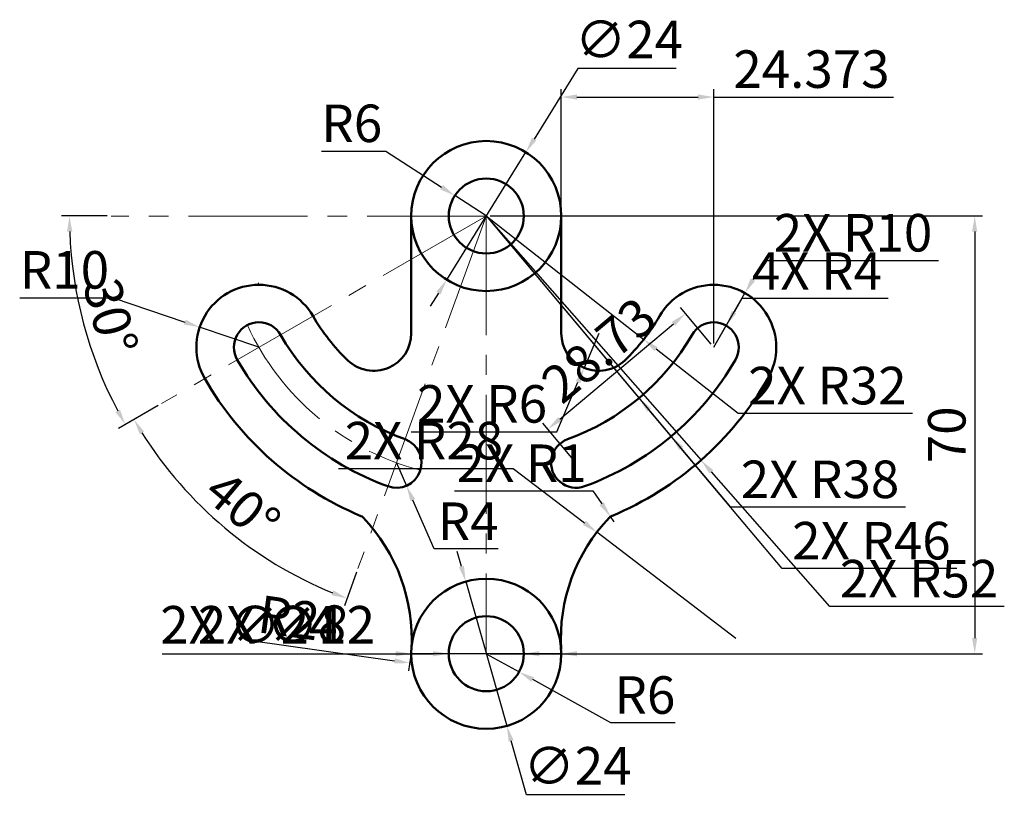
# Model space of a CAD drawing. Units: millimetres. Extents: x 1 to 158, y 37 to 161.
import ezdxf

# ---------------------------------------------------------------- set-up
doc = ezdxf.new("R2010")
doc.units = ezdxf.units.MM
doc.linetypes.add('CENTER2', pattern=[28.575, 19.05, -3.175, 3.175, -3.175])
for name, color, linetype, lineweight in [('M-CNTR', 4, 'CENTER2', 18), ('M-DIMS', 2, 'Continuous', 25), ('M-OUTL', 7, 'Continuous', 50)]:
    doc.layers.add(name, color=color, linetype=linetype, lineweight=lineweight)
doc.styles.get("Standard").update_dxf_attribs({"font": 'arial.ttf'})
doc.dimstyles.new('ISO-25', dxfattribs={"dimtxt": 6, "dimasz": 2.5, "dimexe": 1.25, "dimexo": 0.625, "dimtad": 1, "dimtoh": 1, "dimdec": 0, "dimtxsty": 'Standard', "dimcen": 2.5, "dimadec": 0, "dimazin": 0, "dimtfac": 1, "dimtdec": 0, "dimtmove": 0, "dimatfit": 3, "dimfxl": 1, "dimarcsym": 0})

# ---------------------------------------------------------------- blocks, each defined once
blk = doc.blocks.new('*D1')
at = {"layer": 'Defpoints', "color": 0, "transparency": 16777216}
for p in [(70.21, 133.22), (75.25, 129.97)]:
    blk.add_point(p, dxfattribs=at)
at = {"layer": 'M-DIMS', "color": 0, "lineweight": -2, "transparency": 16777216}
for p, q in [((48.9, 140.32), (59.2, 140.32)), ((59.2, 140.32), (68.11, 134.57)), ((75.25, 129.97), (70.21, 133.22))]:
    blk.add_line(p, q, dxfattribs=at)
at = {"layer": 'M-DIMS', "color": 0, "transparency": 16777216}
blk.add_solid([(68.34, 134.92), (67.89, 134.22), (70.21, 133.22)], dxfattribs=at)
at = {"layer": 'M-DIMS', "color": 0, "transparency": 16777216, "insert": (53.74, 144.01), "char_height": 6, "attachment_point": 5}
blk.add_mtext('R6', dxfattribs=at)
blk = doc.blocks.new('*D2')
at = {"layer": 'Defpoints', "color": 0, "transparency": 16777216}
for p in [(81.59, 140.16), (68.92, 119.77)]:
    blk.add_point(p, dxfattribs=at)
at = {"layer": 'M-DIMS', "color": 0, "lineweight": -2, "transparency": 16777216}
for p, q in [((89.91, 153.57), (82.9, 142.28)), ((105.64, 153.57), (89.91, 153.57)), ((68.92, 119.77), (81.59, 140.16)), ((67.6, 117.65), (66.29, 115.53))]:
    blk.add_line(p, q, dxfattribs=at)
at = {"layer": 'M-DIMS', "color": 0, "transparency": 16777216}
for points in [[(82.55, 142.5), (83.26, 142.06), (81.59, 140.16)], [(67.25, 117.87), (67.96, 117.43), (68.92, 119.77)]]:
    blk.add_solid(points, dxfattribs=at)
at = {"layer": 'M-DIMS', "color": 0, "transparency": 16777216, "insert": (98.09, 157.42), "char_height": 6, "attachment_point": 5}
blk.add_mtext('∅24', dxfattribs=at)
blk = doc.blocks.new('*D3')
at = {"layer": 'Defpoints', "color": 0, "transparency": 16777216}
for p in [(75.25, 129.97), (75.25, 59.97), (153.37, 59.97)]:
    blk.add_point(p, dxfattribs=at)
at = {"layer": 'M-DIMS', "color": 0, "lineweight": -2, "transparency": 16777216}
for p, q in [((75.88, 129.97), (154.62, 129.97)), ((153.37, 127.47), (153.37, 62.47)), ((75.88, 59.97), (154.62, 59.97))]:
    blk.add_line(p, q, dxfattribs=at)
at = {"layer": 'M-DIMS', "color": 0, "transparency": 16777216}
for points in [[(152.95, 127.47), (153.78, 127.47), (153.37, 129.97)], [(152.95, 62.47), (153.78, 62.47), (153.37, 59.97)]]:
    blk.add_solid(points, dxfattribs=at)
at = {"layer": 'M-DIMS', "color": 0, "transparency": 16777216, "insert": (149.68, 94.97), "char_height": 6, "attachment_point": 5, "rotation": 90}
blk.add_mtext('70', dxfattribs=at)
blk = doc.blocks.new('*D4')
at = {"layer": 'Defpoints', "color": 0, "transparency": 16777216}
for p in [(35.33, 62.38), (63.05, 58.48)]:
    blk.add_point(p, dxfattribs=at)
at = {"layer": 'M-DIMS', "color": 0, "lineweight": -2, "transparency": 16777216}
blk.add_line((37.6, 62.06), (60.58, 58.82), dxfattribs=at)
blk.add_arc((35.33, 62.38), 28, 349.422, 355.2587, dxfattribs=at)
at = {"layer": 'M-DIMS', "color": 0, "transparency": 16777216}
blk.add_solid([(60.64, 59.24), (60.52, 58.41), (63.05, 58.48)], dxfattribs=at)
at = {"layer": 'M-DIMS', "color": 0, "transparency": 16777216, "insert": (45.84, 64.63), "char_height": 6, "attachment_point": 5, "rotation": 351.9799}
blk.add_mtext('R28', dxfattribs=at)
blk = doc.blocks.new('*D5')
at = {"layer": 'Defpoints', "color": 0, "transparency": 16777216}
for p in [(29.41, 112.19), (38.88, 108.97)]:
    blk.add_point(p, dxfattribs=at)
at = {"layer": 'M-DIMS', "color": 0, "lineweight": -2, "transparency": 16777216}
for p, q in [((0.63, 116.9), (15.57, 116.9)), ((15.57, 116.9), (27.05, 112.99)), ((38.88, 108.97), (29.41, 112.19))]:
    blk.add_line(p, q, dxfattribs=at)
at = {"layer": 'M-DIMS', "color": 0, "transparency": 16777216}
blk.add_solid([(27.18, 113.39), (26.91, 112.6), (29.41, 112.19)], dxfattribs=at)
at = {"layer": 'M-DIMS', "color": 0, "transparency": 16777216, "insert": (7.79, 120.58), "char_height": 6, "attachment_point": 5}
blk.add_mtext('R10', dxfattribs=at)
blk = doc.blocks.new('*D6')
at = {"layer": 'Defpoints', "color": 0, "transparency": 16777216}
for p in [(60.89, 90.5), (62.49, 86.83)]:
    blk.add_point(p, dxfattribs=at)
at = {"layer": 'M-DIMS', "color": 0, "lineweight": -2, "transparency": 16777216}
for p, q in [((60.89, 90.5), (62.49, 86.83)), ((66.9, 76.76), (63.5, 84.54)), ((77.18, 76.76), (66.9, 76.76))]:
    blk.add_line(p, q, dxfattribs=at)
at = {"layer": 'M-DIMS', "color": 0, "transparency": 16777216}
blk.add_solid([(63.88, 84.71), (63.11, 84.38), (62.49, 86.83)], dxfattribs=at)
at = {"layer": 'M-DIMS', "color": 0, "transparency": 16777216, "insert": (72.35, 80.38), "char_height": 6, "attachment_point": 5}
blk.add_mtext('R4', dxfattribs=at)
blk = doc.blocks.new('*D7')
at = {"layer": 'Defpoints', "color": 0, "transparency": 16777216}
for p in [(75.25, 129.97), (75.25, 129.97), (23.29, 99.97), (27.92, 85.31), (54.73, 73.58)]:
    blk.add_point(p, dxfattribs=at)
at = {"layer": 'M-DIMS', "color": 0, "lineweight": -2, "transparency": 16777216}
for p, q in [((22.75, 99.65), (17.81, 96.8)), ((54.52, 73), (52.57, 67.64))]:
    blk.add_line(p, q, dxfattribs=at)
blk.add_arc((75.25, 129.97), 65.08, 212.2012, 247.7988, dxfattribs=at)
at = {"layer": 'M-DIMS', "color": 0, "transparency": 16777216}
for points in [[(19.83, 95.07), (20.54, 95.5), (18.9, 97.43)], [(50.81, 70.1), (50.51, 69.33), (53, 68.81)]]:
    blk.add_solid(points, dxfattribs=at)
at = {"layer": 'M-DIMS', "color": 0, "transparency": 16777216, "insert": (35.79, 82.94), "char_height": 6, "attachment_point": 5, "rotation": 320}
blk.add_mtext('40°', dxfattribs=at)
blk = doc.blocks.new('*D8')
at = {"layer": 'Defpoints', "color": 0, "transparency": 16777216}
for p in [(15.25, 129.97), (75.25, 129.97), (75.25, 129.97), (9.6, 118.39), (23.29, 99.97)]:
    blk.add_point(p, dxfattribs=at)
at = {"layer": 'M-DIMS', "color": 0, "lineweight": -2, "transparency": 16777216}
for p, q in [((14.63, 129.97), (7.33, 129.97)), ((22.75, 99.65), (16.43, 96.01))]:
    blk.add_line(p, q, dxfattribs=at)
blk.add_arc((75.25, 129.97), 66.67, 182.1486, 207.8514, dxfattribs=at)
at = {"layer": 'M-DIMS', "color": 0, "transparency": 16777216}
for points in [[(8.21, 127.46), (9.05, 127.47), (8.58, 129.97)], [(16.67, 99.02), (15.94, 98.62), (17.52, 96.63)]]:
    blk.add_solid(points, dxfattribs=at)
at = {"layer": 'M-DIMS', "color": 0, "transparency": 16777216, "insert": (14.42, 113.67), "char_height": 6, "attachment_point": 5, "rotation": 285}
blk.add_mtext('30°', dxfattribs=at)
blk = doc.blocks.new('*D9')
at = {"layer": 'Defpoints', "color": 0, "transparency": 16777216}
for p in [(75.25, 59.97), (80.5, 57.05)]:
    blk.add_point(p, dxfattribs=at)
at = {"layer": 'M-DIMS', "color": 0, "lineweight": -2, "transparency": 16777216}
for p, q in [((75.25, 59.97), (80.5, 57.05)), ((95.16, 48.89), (82.68, 55.83)), ((105.46, 48.89), (95.16, 48.89))]:
    blk.add_line(p, q, dxfattribs=at)
at = {"layer": 'M-DIMS', "color": 0, "transparency": 16777216}
blk.add_solid([(82.88, 56.2), (82.48, 55.47), (80.5, 57.05)], dxfattribs=at)
at = {"layer": 'M-DIMS', "color": 0, "transparency": 16777216, "insert": (100.62, 52.58), "char_height": 6, "attachment_point": 5}
blk.add_mtext('R6', dxfattribs=at)
blk = doc.blocks.new('*D10')
at = {"layer": 'Defpoints', "color": 0, "transparency": 16777216}
for p in [(71.96, 71.51), (78.55, 48.43)]:
    blk.add_point(p, dxfattribs=at)
at = {"layer": 'M-DIMS', "color": 0, "lineweight": -2, "transparency": 16777216}
for p, q in [((71.28, 73.91), (70.59, 76.31)), ((71.96, 71.51), (78.55, 48.43)), ((81.69, 37.4), (79.23, 46.02)), ((97.41, 37.4), (81.69, 37.4))]:
    blk.add_line(p, q, dxfattribs=at)
at = {"layer": 'M-DIMS', "color": 0, "transparency": 16777216}
for points in [[(71.68, 74.02), (70.88, 73.8), (71.96, 71.51)], [(79.63, 46.14), (78.83, 45.91), (78.55, 48.43)]]:
    blk.add_solid(points, dxfattribs=at)
at = {"layer": 'M-DIMS', "color": 0, "transparency": 16777216, "insert": (89.86, 41.26), "char_height": 6, "attachment_point": 5}
blk.add_mtext('∅24', dxfattribs=at)
blk = doc.blocks.new('HUB-OD24-BORE12')
for radius in [12, 6]:
    blk.add_circle((12, 12), radius)
blk = doc.blocks.new('*D12')
at = {"layer": 'Defpoints', "color": 0, "transparency": 16777216}
for p in [(111.63, 148.99), (87.25, 111.2), (111.63, 108.97)]:
    blk.add_point(p, dxfattribs=at)
at = {"layer": 'M-DIMS', "color": 0, "lineweight": -2, "transparency": 16777216}
for p, q in [((87.25, 111.83), (87.25, 150.24)), ((111.63, 109.59), (111.63, 150.24)), ((89.75, 148.99), (109.13, 148.99)), ((111.63, 148.99), (140.39, 148.99))]:
    blk.add_line(p, q, dxfattribs=at)
at = {"layer": 'M-DIMS', "color": 0, "transparency": 16777216}
for points in [[(89.75, 149.41), (89.75, 148.57), (87.25, 148.99)], [(109.13, 149.41), (109.13, 148.57), (111.63, 148.99)]]:
    blk.add_solid(points, dxfattribs=at)
at = {"layer": 'M-DIMS', "color": 0, "transparency": 16777216, "insert": (127.26, 152.68), "char_height": 6, "attachment_point": 5}
blk.add_mtext('24.373', dxfattribs=at)
blk = doc.blocks.new('*D13')
at = {"layer": 'Defpoints', "color": 0, "transparency": 16777216}
for p in [(107.11, 114.35), (111.63, 108.97), (89.62, 90.5)]:
    blk.add_point(p, dxfattribs=at)
at = {"layer": 'M-DIMS', "color": 0, "lineweight": -2, "transparency": 16777216}
for p, q in [((111.23, 109.45), (106.31, 115.31)), ((87.02, 97.49), (105.2, 112.74)), ((89.22, 90.98), (84.3, 96.84))]:
    blk.add_line(p, q, dxfattribs=at)
at = {"layer": 'M-DIMS', "color": 0, "transparency": 16777216}
for points in [[(104.93, 113.06), (105.46, 112.42), (107.11, 114.35)], [(86.75, 97.81), (87.29, 97.17), (85.1, 95.88)]]:
    blk.add_solid(points, dxfattribs=at)
at = {"layer": 'M-DIMS', "color": 0, "transparency": 16777216, "insert": (93.74, 107.94), "char_height": 6, "attachment_point": 5, "rotation": 40}
blk.add_mtext('28.73', dxfattribs=at)
blk = doc.blocks.new('*D14')
at = {"layer": 'Defpoints', "color": 0, "transparency": 16777216}
for p in [(75.25, 129.97), (109.6, 90.92)]:
    blk.add_point(p, dxfattribs=at)
at = {"layer": 'M-DIMS', "color": 0, "lineweight": -2, "transparency": 16777216}
for p, q in [((75.25, 129.97), (109.6, 90.92)), ((130.21, 67.5), (111.25, 89.05)), ((158.1, 67.5), (130.21, 67.5))]:
    blk.add_line(p, q, dxfattribs=at)
at = {"layer": 'M-DIMS', "color": 0, "transparency": 16777216}
blk.add_solid([(111.57, 89.32), (110.94, 88.77), (109.6, 90.92)], dxfattribs=at)
at = {"layer": 'M-DIMS', "color": 0, "transparency": 16777216, "insert": (144.47, 71.19), "char_height": 6, "attachment_point": 5}
blk.add_mtext('2X R52', dxfattribs=at)
blk = doc.blocks.new('*D15')
at = {"layer": 'Defpoints', "color": 0, "transparency": 16777216}
for p in [(75.25, 129.97), (104.82, 94.73)]:
    blk.add_point(p, dxfattribs=at)
at = {"layer": 'M-DIMS', "color": 0, "lineweight": -2, "transparency": 16777216}
for p, q in [((75.25, 129.97), (104.82, 94.73)), ((122.56, 73.59), (106.43, 92.81)), ((150.52, 73.59), (122.56, 73.59))]:
    blk.add_line(p, q, dxfattribs=at)
at = {"layer": 'M-DIMS', "color": 0, "transparency": 16777216}
blk.add_solid([(106.75, 93.08), (106.11, 92.55), (104.82, 94.73)], dxfattribs=at)
at = {"layer": 'M-DIMS', "color": 0, "transparency": 16777216, "insert": (136.85, 77.27), "char_height": 6, "attachment_point": 5}
blk.add_mtext('2X R46', dxfattribs=at)
blk = doc.blocks.new('*D16')
at = {"layer": 'Defpoints', "color": 0, "transparency": 16777216}
for p in [(75.25, 129.97), (99.68, 100.86)]:
    blk.add_point(p, dxfattribs=at)
at = {"layer": 'M-DIMS', "color": 0, "lineweight": -2, "transparency": 16777216}
for p, q in [((75.25, 129.97), (99.68, 100.86)), ((114.34, 83.39), (101.29, 98.94)), ((142.3, 83.39), (114.34, 83.39))]:
    blk.add_line(p, q, dxfattribs=at)
at = {"layer": 'M-DIMS', "color": 0, "transparency": 16777216}
blk.add_solid([(101.61, 99.21), (100.97, 98.67), (99.68, 100.86)], dxfattribs=at)
at = {"layer": 'M-DIMS', "color": 0, "transparency": 16777216, "insert": (128.63, 87.08), "char_height": 6, "attachment_point": 5}
blk.add_mtext('2X R38', dxfattribs=at)
blk = doc.blocks.new('*D17')
at = {"layer": 'Defpoints', "color": 0, "transparency": 16777216}
for p in [(75.25, 129.97), (100.44, 110.22)]:
    blk.add_point(p, dxfattribs=at)
at = {"layer": 'M-DIMS', "color": 0, "lineweight": -2, "transparency": 16777216}
for p, q in [((75.25, 129.97), (100.44, 110.22)), ((115.55, 98.38), (102.41, 108.68)), ((143.44, 98.38), (115.55, 98.38))]:
    blk.add_line(p, q, dxfattribs=at)
at = {"layer": 'M-DIMS', "color": 0, "transparency": 16777216}
blk.add_solid([(102.66, 109.01), (102.15, 108.35), (100.44, 110.22)], dxfattribs=at)
at = {"layer": 'M-DIMS', "color": 0, "transparency": 16777216, "insert": (129.81, 102.07), "char_height": 6, "attachment_point": 5}
blk.add_mtext('2X R32', dxfattribs=at)
blk = doc.blocks.new('*D18')
at = {"layer": 'Defpoints', "color": 0, "transparency": 16777216}
for p in [(92.93, 79.38), (115.18, 62.38)]:
    blk.add_point(p, dxfattribs=at)
at = {"layer": 'M-DIMS', "color": 0, "lineweight": -2, "transparency": 16777216}
for p, q in [((51.61, 89.58), (79.58, 89.58)), ((79.58, 89.58), (90.94, 80.9)), ((115.18, 62.38), (92.93, 79.38))]:
    blk.add_line(p, q, dxfattribs=at)
at = {"layer": 'M-DIMS', "color": 0, "transparency": 16777216}
blk.add_solid([(91.2, 81.23), (90.69, 80.57), (92.93, 79.38)], dxfattribs=at)
at = {"layer": 'M-DIMS', "color": 0, "transparency": 16777216, "insert": (65.28, 93.27), "char_height": 6, "attachment_point": 5}
blk.add_mtext('2X R28', dxfattribs=at)
blk = doc.blocks.new('*D19')
at = {"layer": 'Defpoints', "color": 0, "transparency": 16777216}
for p in [(63.25, 59.97), (87.25, 59.97)]:
    blk.add_point(p, dxfattribs=at)
at = {"layer": 'M-DIMS', "color": 0, "lineweight": -2, "transparency": 16777216}
for p, q in [((23.39, 59.97), (51.79, 59.97)), ((51.79, 59.97), (60.75, 59.97)), ((87.25, 59.97), (63.25, 59.97)), ((89.75, 59.97), (92.25, 59.97))]:
    blk.add_line(p, q, dxfattribs=at)
at = {"layer": 'M-DIMS', "color": 0, "transparency": 16777216}
for points in [[(60.75, 60.38), (60.75, 59.55), (63.25, 59.97)], [(89.75, 60.38), (89.75, 59.55), (87.25, 59.97)]]:
    blk.add_solid(points, dxfattribs=at)
at = {"layer": 'M-DIMS', "color": 0, "transparency": 16777216, "insert": (37.28, 63.82), "char_height": 6, "attachment_point": 5}
blk.add_mtext('2X ∅24', dxfattribs=at)
blk = doc.blocks.new('*D20')
at = {"layer": 'Defpoints', "color": 0, "transparency": 16777216}
for p in [(69.25, 59.97), (81.25, 59.97)]:
    blk.add_point(p, dxfattribs=at)
at = {"layer": 'M-DIMS', "color": 0, "lineweight": -2, "transparency": 16777216}
for p, q in [((29.43, 59.97), (57.79, 59.97)), ((57.79, 59.97), (66.75, 59.97)), ((81.25, 59.97), (69.25, 59.97)), ((83.75, 59.97), (86.25, 59.97))]:
    blk.add_line(p, q, dxfattribs=at)
at = {"layer": 'M-DIMS', "color": 0, "transparency": 16777216}
for points in [[(66.75, 60.38), (66.75, 59.55), (69.25, 59.97)], [(83.75, 60.38), (83.75, 59.55), (81.25, 59.97)]]:
    blk.add_solid(points, dxfattribs=at)
at = {"layer": 'M-DIMS', "color": 0, "transparency": 16777216, "insert": (43.3, 63.82), "char_height": 6, "attachment_point": 5}
blk.add_mtext('2X ∅12', dxfattribs=at)
blk = doc.blocks.new('*D21')
at = {"layer": 'Defpoints', "color": 0, "transparency": 16777216}
for p in [(116.63, 117.63), (111.63, 108.97)]:
    blk.add_point(p, dxfattribs=at)
at = {"layer": 'M-DIMS', "color": 0, "lineweight": -2, "transparency": 16777216}
for p, q in [((119.63, 122.82), (117.88, 119.79)), ((147.56, 122.82), (119.63, 122.82)), ((111.63, 108.97), (116.63, 117.63))]:
    blk.add_line(p, q, dxfattribs=at)
at = {"layer": 'M-DIMS', "color": 0, "transparency": 16777216}
blk.add_solid([(117.52, 120), (118.24, 119.58), (116.63, 117.63)], dxfattribs=at)
at = {"layer": 'M-DIMS', "color": 0, "transparency": 16777216, "insert": (133.91, 126.51), "char_height": 6, "attachment_point": 5}
blk.add_mtext('2X R10', dxfattribs=at)
blk = doc.blocks.new('*D22')
at = {"layer": 'Defpoints', "color": 0, "transparency": 16777216}
for p in [(93.25, 111.2), (90.9, 105.69)]:
    blk.add_point(p, dxfattribs=at)
at = {"layer": 'M-DIMS', "color": 0, "lineweight": -2, "transparency": 16777216}
for p, q in [((93.25, 111.2), (90.9, 105.69)), ((86.54, 95.45), (89.92, 103.39)), ((63.25, 95.45), (86.54, 95.45))]:
    blk.add_line(p, q, dxfattribs=at)
at = {"layer": 'M-DIMS', "color": 0, "transparency": 16777216}
blk.add_solid([(89.54, 103.55), (90.3, 103.22), (90.9, 105.69)], dxfattribs=at)
at = {"layer": 'M-DIMS', "color": 0, "transparency": 16777216, "insert": (74.58, 99.14), "char_height": 6, "attachment_point": 5}
blk.add_mtext('2X R6', dxfattribs=at)
blk = doc.blocks.new('*D23')
at = {"layer": 'Defpoints', "color": 0, "transparency": 16777216}
for p in [(113.63, 112.43), (111.63, 108.97)]:
    blk.add_point(p, dxfattribs=at)
at = {"layer": 'M-DIMS', "color": 0, "lineweight": -2, "transparency": 16777216}
for p, q in [((116.13, 116.76), (114.88, 114.6)), ((139.54, 116.76), (116.13, 116.76)), ((111.63, 108.97), (113.63, 112.43))]:
    blk.add_line(p, q, dxfattribs=at)
at = {"layer": 'M-DIMS', "color": 0, "transparency": 16777216}
blk.add_solid([(114.52, 114.8), (115.24, 114.39), (113.63, 112.43)], dxfattribs=at)
at = {"layer": 'M-DIMS', "color": 0, "transparency": 16777216, "insert": (128.14, 120.39), "char_height": 6, "attachment_point": 5}
blk.add_mtext('4X R4', dxfattribs=at)
blk = doc.blocks.new('*D24')
at = {"layer": 'Defpoints', "color": 0, "transparency": 16777216}
for p in [(95.12, 81.89), (95.69, 81.06)]:
    blk.add_point(p, dxfattribs=at)
at = {"layer": 'M-DIMS', "color": 0, "lineweight": -2, "transparency": 16777216}
for p, q in [((70.16, 86.01), (92.29, 86.01)), ((92.29, 86.01), (93.71, 83.95)), ((95.69, 81.06), (95.12, 81.89))]:
    blk.add_line(p, q, dxfattribs=at)
at = {"layer": 'M-DIMS', "color": 0, "transparency": 16777216}
blk.add_solid([(94.05, 84.19), (93.36, 83.71), (95.12, 81.89)], dxfattribs=at)
at = {"layer": 'M-DIMS', "color": 0, "transparency": 16777216, "insert": (80.91, 89.65), "char_height": 6, "attachment_point": 5}
blk.add_mtext('2X R1', dxfattribs=at)

msp = doc.modelspace()

# ---------------------------------------------------------------- linework, layer by layer
at = {"layer": 'M-CNTR'}
for q in [(15.2544, 129.9664), (23.2929, 99.9664), (54.7332, 73.5848), (75.2544, 59.9664)]:
    msp.add_line((75.2544, 129.9664), q, dxfattribs=at)
for radius, start, end in [(38, 196.325718, 196.826449), (42, 204.541195, 255.458805)]:
    msp.add_arc((75.2544, 129.9664), radius, start, end, dxfattribs=at)
at = {"layer": 'M-OUTL'}
for points in [[(63.2763, 60.6911, 0.20911078), (55.5429, 81.7556, 0.10308155), (55.2065, 81.9864, -0.16430715), (30.2211, 103.9664, -1), (47.5416, 113.9664, 0.07074652), (53.1006, 106.8751, 0.66071318), (63.2544, 111.2047), (63.2544, 129.9664)], [(87.2325, 60.6911, -0.20911078), (94.9659, 81.7556, -0.10308155), (95.3023, 81.9864, 0.16430715), (120.2877, 103.9664, 1), (102.9672, 113.9664, -0.07074652), (97.4083, 106.8751, -0.66071318), (87.2544, 111.2047), (87.2544, 129.9664)]]:
    msp.add_lwpolyline(points, format="xyb", dxfattribs=at)
for points in [[(42.3454, 110.9664, 1), (35.4172, 106.9664, 0.17632698), (59.5215, 86.7405, 1), (62.2576, 94.2581, -0.17632698)], [(108.1634, 110.9664, -1), (115.0916, 106.9664, -0.17632698), (90.9873, 86.7405, -1), (88.2512, 94.2581, 0.17632698)]]:
    msp.add_lwpolyline(points, format="xyb", close=True, dxfattribs=at)

# ---------------------------------------------------------------- block references
for p in [(63.254, 117.966), (63.254, 47.966)]:
    msp.add_blockref('HUB-OD24-BORE12', p, dxfattribs=at)

# ---------------------------------------------------------------- dimensions: what is measured, and where the dimension line sits
at = {"layer": 'M-DIMS'}
dim = msp.add_diameter_dim_2p(p1=(68.9232, 119.7725), p2=(81.5856, 140.1603), dimstyle='ISO-25', override={"dimclrd": 0, "dimclre": 0, "dimclrt": 0}, dxfattribs=at)
dim.commit()
dim.dimension.update_dxf_attribs({"geometry": '*D2', "text_midpoint": (98.0868, 153.5676), "dimtype": 163})
dim = msp.add_linear_dim(base=(111.6275, 148.9914), p1=(87.2544, 111.2047), p2=(111.6275, 108.9664), dimstyle='ISO-25', override={"dimdec": 3, "dimlfac": 1, "dimrnd": 0, "dimzin": 0, "dimdsep": 46, "dimlunit": 2}, dxfattribs=at)
dim.commit()
dim.dimension.update_dxf_attribs({"geometry": '*D12', "text_midpoint": (127.2579, 152.6819)})
for center, mpoint, picture, middle in [((75.2544, 129.9664), (70.212, 133.2182), '*D1', (53.738, 140.3206)), ((38.8813, 108.9664), (29.4141, 112.1869), '*D5', (7.7879, 116.8961)), ((35.3274, 62.3821), (63.0536, 58.4755), '*D4', (45.3264, 60.9732)), ((75.2544, 59.9664), (80.4973, 57.0488), '*D9', (100.6245, 48.8869))]:
    dim = msp.add_radius_dim(center=center, mpoint=mpoint, dimstyle='ISO-25', override={"dimclrd": 0, "dimclre": 0, "dimclrt": 0}, dxfattribs=at)
    dim.commit()
    dim.dimension.update_dxf_attribs({"geometry": picture, "text_midpoint": middle, "dimtype": 164})
for center, mpoint, picture, middle in [((111.6275, 108.9664), (116.627, 117.6269), '*D21', (133.9072, 122.8233)), ((75.2544, 129.9664), (109.601, 90.924), '*D14', (144.4691, 67.4985)), ((75.2544, 129.9664), (104.8227, 94.7284), '*D15', (136.8524, 73.5856)), ((75.2544, 129.9664), (99.6803, 100.8567), '*D16', (128.6327, 83.3908)), ((75.2544, 129.9664), (100.4387, 110.2242), '*D17', (129.8093, 98.379)), ((115.1814, 62.3821), (92.9307, 79.3793), '*D18', (65.2834, 89.5777))]:
    dim = msp.add_radius_dim(center=center, mpoint=mpoint, text='2X <>', dimstyle='ISO-25', override={"dimdec": 0, "dimlfac": 1, "dimrnd": 0, "dimzin": 0, "dimdsep": 46, "dimlunit": 2}, dxfattribs=at)
    dim.commit()
    dim.dimension.update_dxf_attribs({"geometry": picture, "text_midpoint": middle, "dimtype": 164})
for base, line2, picture, middle in [((9.5966, 118.3891), ((75.2544, 129.9664), (15.2544, 129.9664)), '*D8', (14.4202, 113.6659)), ((27.9191, 85.3078), ((75.2544, 129.9664), (54.7332, 73.5848)), '*D7', (35.7946, 82.94))]:
    dim = msp.add_angular_dim_2l(base=base, line1=((75.2544, 129.9664), (23.2929, 99.9664)), line2=line2, dimstyle='ISO-25', override={"dimclrd": 0, "dimclre": 0, "dimclrt": 0}, dxfattribs=at)
    dim.commit()
    dim.dimension.update_dxf_attribs({"geometry": picture, "text_midpoint": middle})
for base, p1, p2, angle, override, picture, middle in [((153.3664, 59.9664), (75.2544, 129.9664), (75.2544, 59.9664), 90, {"dimclrd": 0, "dimclre": 0, "dimclrt": 0}, '*D3', (149.678, 94.9664)), ((107.1119, 114.3478), (89.6192, 90.4993), (111.6275, 108.9664), 40, {"dimdec": 2, "dimlfac": 1, "dimrnd": 0, "dimzin": 0, "dimdsep": 46, "dimlunit": 2}, '*D13', (93.7356, 107.9414))]:
    dim = msp.add_linear_dim(base=base, p1=p1, p2=p2, angle=angle, dimstyle='ISO-25', override=override, dxfattribs=at)
    dim.commit()
    dim.dimension.update_dxf_attribs({"geometry": picture, "text_midpoint": middle})
for center, mpoint, text, picture, middle in [((111.6275, 108.9664), (113.6273, 112.4306), '4X <>', '*D23', (128.1444, 120.3878)), ((93.2544, 111.2047), (90.9008, 105.6856), '2X <>', '*D22', (74.5783, 99.1389)), ((95.6878, 81.0637), (95.1219, 81.8881), '2X <>', '*D24', (80.9115, 89.6497))]:
    dim = msp.add_radius_dim(center=center, mpoint=mpoint, text=text, dimstyle='ISO-25', override={"dimdec": 0, "dimlfac": 1, "dimrnd": 0, "dimzin": 0, "dimdsep": 46, "dimlunit": 2}, dxfattribs=at)
    dim.commit()
    dim.dimension.update_dxf_attribs({"geometry": picture, "text_midpoint": middle})
dim = msp.add_radius_dim(center=(60.8896, 90.4993), mpoint=(62.4935, 86.8349), dimstyle='ISO-25', override={"dimclrd": 0, "dimclre": 0, "dimclrt": 0}, dxfattribs=at)
dim.commit()
dim.dimension.update_dxf_attribs({"geometry": '*D6', "text_midpoint": (72.3546, 80.383)})
dim = msp.add_diameter_dim_2p(p1=(71.9628, 71.5061), p2=(78.546, 48.4267), dimstyle='ISO-25', override={"dimclrd": 0, "dimclre": 0, "dimclrt": 0}, dxfattribs=at)
dim.commit()
dim.dimension.update_dxf_attribs({"geometry": '*D10', "text_midpoint": (89.8643, 41.2601)})
for p1, p2, picture, middle in [((87.2544, 59.9668), (63.2544, 59.966), '*D19', (51.7919, 59.9656)), ((81.2544, 59.9668), (69.2544, 59.966), '*D20', (57.7919, 59.9653))]:
    dim = msp.add_diameter_dim_2p(p1=p1, p2=p2, text='2X <>', dimstyle='ISO-25', override={"dimdec": 0, "dimlfac": 1, "dimrnd": 0, "dimzin": 0, "dimdsep": 46, "dimlunit": 2}, dxfattribs=at)
    dim.commit()
    dim.dimension.update_dxf_attribs({"geometry": picture, "text_midpoint": middle})

doc.saveas('drawing.dxf')
